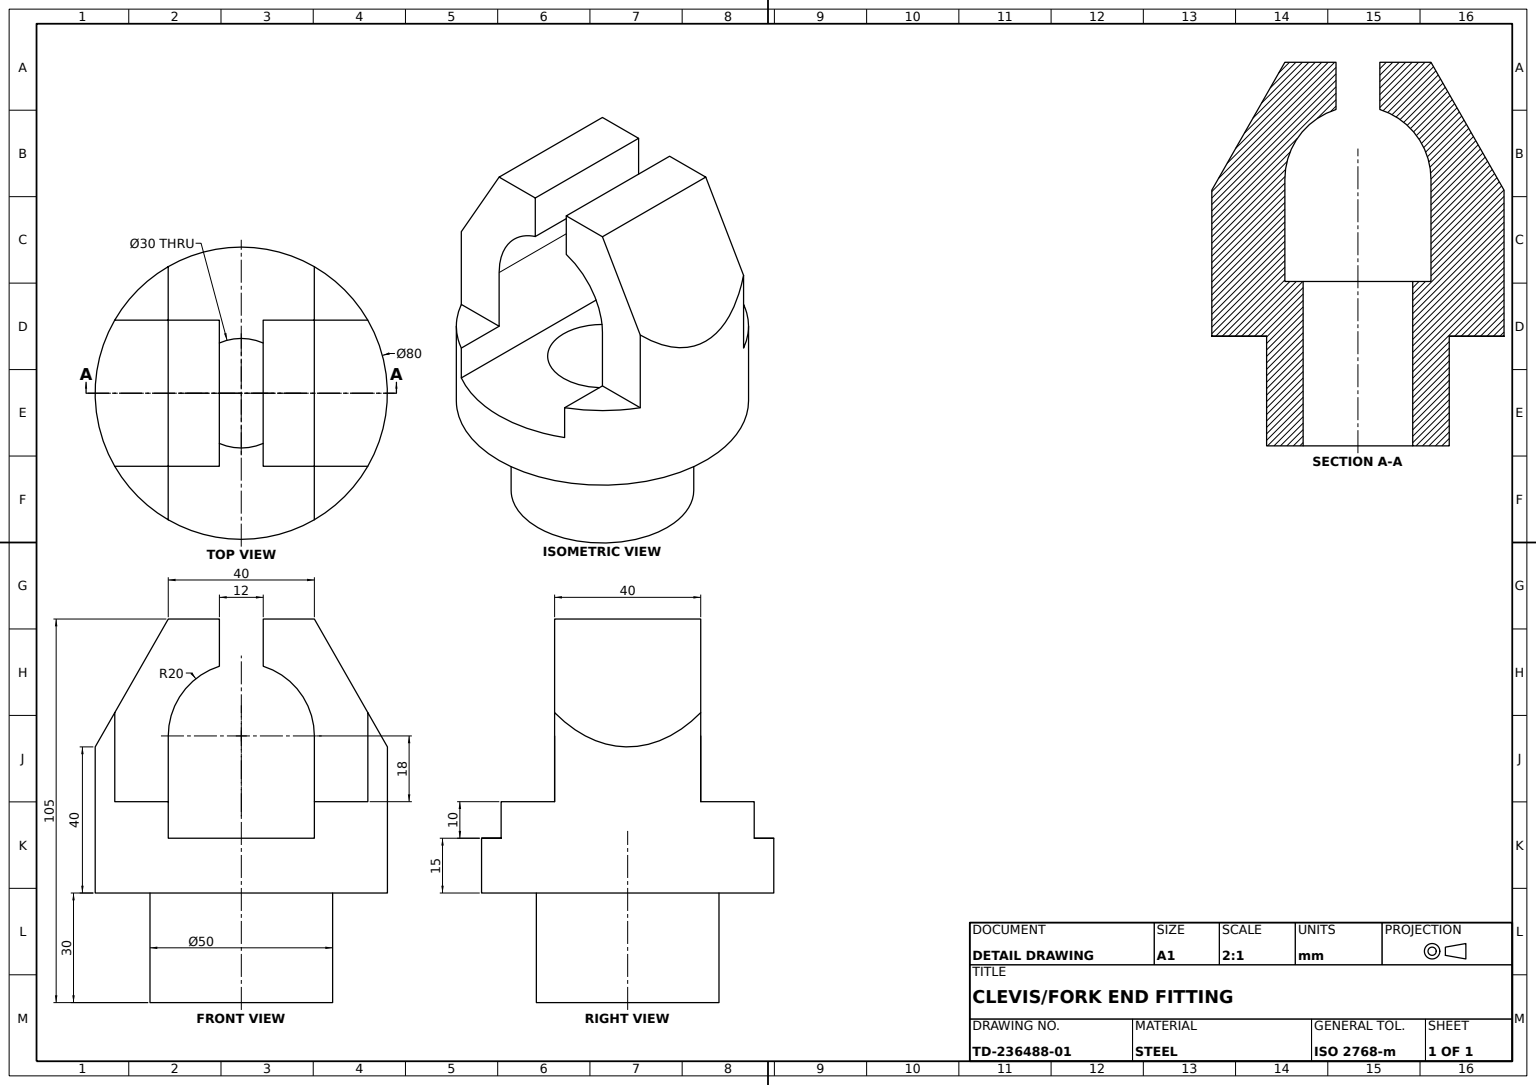
SolidWorks part; units mm, degrees
material "Plain Carbon Steel"
ref_plane "Front Plane" through (0, 0, 0) normal (0, 0, 1) x (1, 0, 0)
ref_plane "Top Plane" through (0, 0, 0) normal (0, 1, 0) x (1, 0, 0)
ref_plane "Right Plane" through (0, 0, 0) normal (1, 0, 0) x (0, 0, -1)
sketch "Body Profile Sketch" plane through (0, 0, 0) normal (0, 0, 1) x (1, 0, 0)
  line L0 (15, 0) -> (25, 0)
  line L1 (25, 0) -> (25, 30)
  line L2 (25, 30) -> (40, 30)
  line L3 (40, 30) -> (40, 105)
  line L4 (40, 105) -> (0, 105)
  line L6 (0, 0) -> (0, 66.8052) construction
  line L7 (0, 105) -> (0, 55)
  line L8 (0, 55) -> (15, 55)
  line L9 (15, 55) -> (15, 0)
  dimension "D1" = 50
  dimension "D2" = 25
  dimension "D3" = 40
  dimension "D4" = 105
  dimension "D5" = 30
  dimension "D6" = 15
revolve "Revolved Body" add sketch "Body Profile Sketch" angle 360 about L6
sketch "Fork Side Profile Sketch" plane through (0, 0, 0) normal (1, 0, 0) x (0, 0, -1)
  line L0 (0, 0) -> (0, 26.676) construction
  line L1 (-40, 105) -> (-20, 105)
  line L2 (-40, 105) -> (-40, 55)
  line L3 (-40, 55) -> (-20, 55)
  line L4 (-20, 105) -> (-20, 55)
  line L5 (40, 105) -> (20, 105)
  line L6 (40, 105) -> (40, 55)
  line L7 (40, 55) -> (20, 55)
  line L8 (20, 105) -> (20, 55)
  line L9 (-25, 0) -> (25, 0) construction
  dimension "D1" = 50
  dimension "D2" = 40
extrude "Fork Side Profile Cut" cut sketch "Fork Side Profile Sketch" against normal through all both and the other way through all
sketch "Fork Slot Sketch" plane through (0, 0, 0) normal (0, 0, 1) x (1, 0, 0)
  line L0 (-40, 105) -> (-20, 105)
  line L1 (34.641, 105) -> (-34.641, 105) construction
  line L2 (-20, 105) -> (-40, 70)
  line L3 (-40, 105) -> (-40, 30) construction
  line L4 (-40, 70) -> (-40, 105)
  line L5 (0, 0) -> (0, 21.9218) construction
  line L6 (40, 105) -> (20, 105)
  line L7 (40, 70) -> (40, 105)
  line L8 (20, 105) -> (40, 70)
  line L9 (34.641, 55) -> (-34.641, 55) construction
  line L10 (-20, 45) -> (20, 45)
  line L11 (-20, 45) -> (-20, 73)
  line L13 (20, 45) -> (20, 73)
  line L15 (-6, 105) -> (-6, 92.0788)
  line L16 (6, 105) -> (6, 92.0788)
  line L17 (-6, 105) -> (6, 105)
  arc A0 (-20, 73) -> (-6, 92.0788) centre (0, 73) cw
  arc A1 (6, 92.0788) -> (20, 73) centre (0, 73) cw
  point P20 (0, 45)
  dimension "D5" = 18
  dimension "D1" = 20
  dimension "D2" = 70
  dimension "D3" = 10
  dimension "D4" = 40
  dimension "D6" = 12
extrude "Fork Slot Cut" cut sketch "Fork Slot Sketch" against normal through all both and the other way through all
